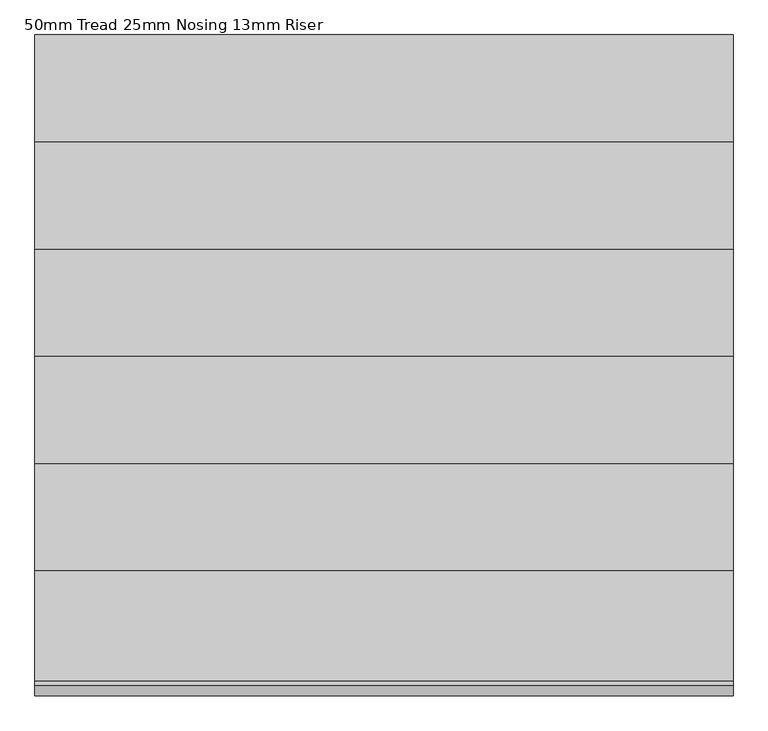
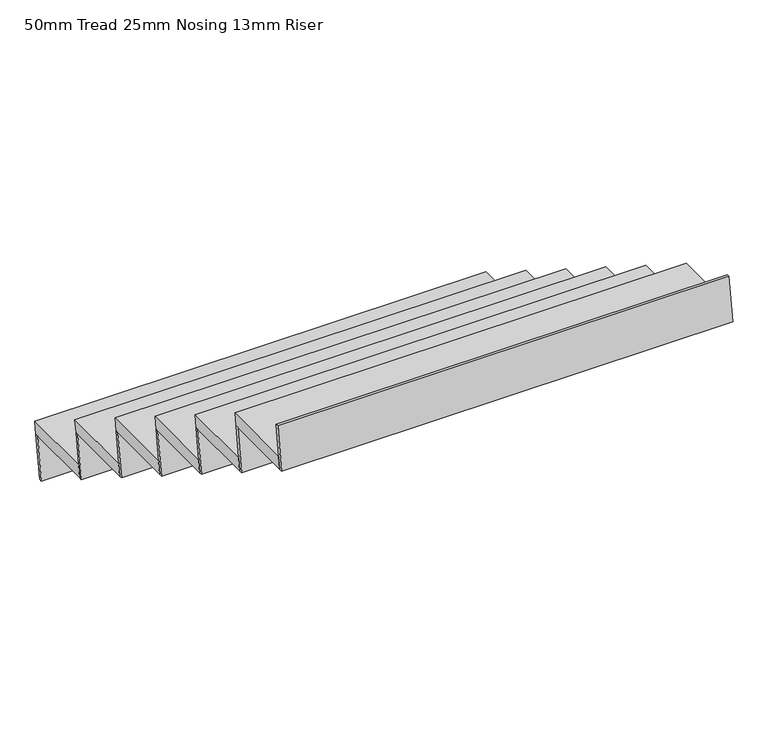
"""IFC4 building model written with IfcOpenShell, lengths in millimetres: stair flight geometry, 50mm Tread 25mm Nosing 13mm Riser."""

from ifc_helpers import new_model, si_unit, frame, origin, place, context, project, spatial, polyline, outline, extrude, source, transform, mapped, element, save


def stair_flight_50mm_tread_25mm_nosing_13mm_riser_6e0c1f45(model_context):
    return source(origin(), model_context, "Body", "SweptSolid", [
        extrude(outline(polyline([(10092.1981148, 1391.3043478), (10392.1981148, 1391.3043478), (10385.0106148, 1341.3043478), (10085.0106148, 1341.3043478), (10092.1981148, 1391.3043478)])), frame((466.2714992, 0.0, 0.0), z_axis=(1.0, 0.0, 0.0), x_axis=(0.0, 1.0, 0.0)), (0.0, 0.0, 1.0), 1789.4101574),
        extrude(outline(polyline([(10385.0106148, 1341.3043478), (10360.0106148, 1167.3913043), (10347.3821248, 1167.3913043), (10372.3821248, 1341.3043478), (10385.0106148, 1341.3043478)])), frame((466.2714992, 0.0, 0.0), z_axis=(1.0, 0.0, 0.0), x_axis=(0.0, 1.0, 0.0)), (0.0, 0.0, 1.0), 1789.4101574),
        extrude(outline(polyline([(10110.0106148, 1515.2173913), (10085.0106148, 1341.3043478), (10072.3821248, 1341.3043478), (10097.3821248, 1515.2173913), (10110.0106148, 1515.2173913)])), frame((466.2714992, 0.0, 0.0), z_axis=(1.0, 0.0, 0.0), x_axis=(0.0, 1.0, 0.0)), (0.0, 0.0, 1.0), 1789.4101574),
        extrude(outline(polyline([(9817.1981148, 1565.2173913), (10117.1981148, 1565.2173913), (10110.0106148, 1515.2173913), (9810.0106148, 1515.2173913), (9817.1981148, 1565.2173913)])), frame((466.2714992, 0.0, 0.0), z_axis=(1.0, 0.0, 0.0), x_axis=(0.0, 1.0, 0.0)), (0.0, 0.0, 1.0), 1789.4101574),
        extrude(outline(polyline([(9835.0106148, 1689.1304348), (9810.0106148, 1515.2173913), (9797.3821248, 1515.2173913), (9822.3821248, 1689.1304348), (9835.0106148, 1689.1304348)])), frame((466.2714992, 0.0, 0.0), z_axis=(1.0, 0.0, 0.0), x_axis=(0.0, 1.0, 0.0)), (0.0, 0.0, 1.0), 1789.4101574),
        extrude(outline(polyline([(9542.1981148, 1739.1304348), (9842.1981148, 1739.1304348), (9835.0106148, 1689.1304348), (9535.0106148, 1689.1304348), (9542.1981148, 1739.1304348)])), frame((466.2714992, 0.0, 0.0), z_axis=(1.0, 0.0, 0.0), x_axis=(0.0, 1.0, 0.0)), (0.0, 0.0, 1.0), 1789.4101574),
        extrude(outline(polyline([(9560.0106148, 1863.0434783), (9535.0106148, 1689.1304348), (9522.3821248, 1689.1304348), (9547.3821248, 1863.0434783), (9560.0106148, 1863.0434783)])), frame((466.2714992, 0.0, 0.0), z_axis=(1.0, 0.0, 0.0), x_axis=(0.0, 1.0, 0.0)), (0.0, 0.0, 1.0), 1789.4101574),
        extrude(outline(polyline([(9267.1981148, 1913.0434783), (9567.1981148, 1913.0434783), (9560.0106148, 1863.0434783), (9260.0106148, 1863.0434783), (9267.1981148, 1913.0434783)])), frame((466.2714992, 0.0, 0.0), z_axis=(1.0, 0.0, 0.0), x_axis=(0.0, 1.0, 0.0)), (0.0, 0.0, 1.0), 1789.4101574),
        extrude(outline(polyline([(9285.0106148, 2036.9565217), (9260.0106148, 1863.0434783), (9247.3821248, 1863.0434783), (9272.3821248, 2036.9565217), (9285.0106148, 2036.9565217)])), frame((466.2714992, 0.0, 0.0), z_axis=(1.0, 0.0, 0.0), x_axis=(0.0, 1.0, 0.0)), (0.0, 0.0, 1.0), 1789.4101574),
        extrude(outline(polyline([(8992.1981148, 2086.9565217), (9292.1981148, 2086.9565217), (9285.0106148, 2036.9565217), (8985.0106148, 2036.9565217), (8992.1981148, 2086.9565217)])), frame((466.2714992, 0.0, 0.0), z_axis=(1.0, 0.0, 0.0), x_axis=(0.0, 1.0, 0.0)), (0.0, 0.0, 1.0), 1789.4101574),
        extrude(outline(polyline([(9010.0106148, 2210.8695652), (8985.0106148, 2036.9565217), (8972.3821248, 2036.9565217), (8997.3821248, 2210.8695652), (9010.0106148, 2210.8695652)])), frame((466.2714992, 0.0, 0.0), z_axis=(1.0, 0.0, 0.0), x_axis=(0.0, 1.0, 0.0)), (0.0, 0.0, 1.0), 1789.4101574),
        extrude(outline(polyline([(8735.0106148, 2384.7826087), (8710.0106148, 2210.8695652), (8697.3821248, 2210.8695652), (8722.3821248, 2384.7826087), (8735.0106148, 2384.7826087)])), frame((466.2714992, 0.0, 0.0), z_axis=(1.0, 0.0, 0.0), x_axis=(0.0, 1.0, 0.0)), (0.0, 0.0, 1.0), 1789.4101574),
        extrude(outline(polyline([(8717.1981148, 2260.8695652), (9017.1981148, 2260.8695652), (9010.0106148, 2210.8695652), (8710.0106148, 2210.8695652), (8717.1981148, 2260.8695652)])), frame((466.2714992, 0.0, 0.0), z_axis=(1.0, 0.0, 0.0), x_axis=(0.0, 1.0, 0.0)), (0.0, 0.0, 1.0), 1789.4101574),
    ])


if __name__ == "__main__":
    model = new_model("IFC4")
    model_context = context("Model", 3, world=origin())
    ifc_project = project(units=[si_unit("LENGTHUNIT", "METRE", prefix="MILLI")], contexts=[model_context])
    site = spatial("IfcSite", under=ifc_project)
    building = spatial("IfcBuilding", under=site)
    placement = place(None, origin())
    stair_flight_50mm_tread_25mm_nosing_13mm_riser_shape = stair_flight_50mm_tread_25mm_nosing_13mm_riser_6e0c1f45(model_context)
    element("IfcStairFlight", 1, ObjectType="50mm Tread 25mm Nosing 13mm Riser", at=placement, inside=building, context=model_context, shape_type="MappedRepresentation", body=[
        mapped(stair_flight_50mm_tread_25mm_nosing_13mm_riser_shape, transform((0.0, 0.0, 0.0), x_axis=(1.0, 0.0, 0.0), y_axis=(0.0, 1.0, 0.0), z_axis=(0.0, 0.0, 1.0))),
    ])
    save(model, "model.ifc")
